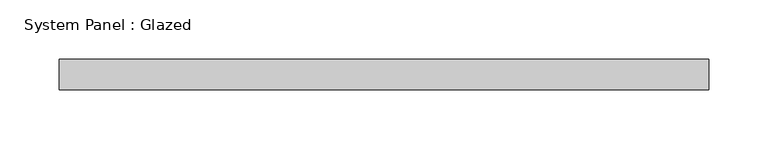
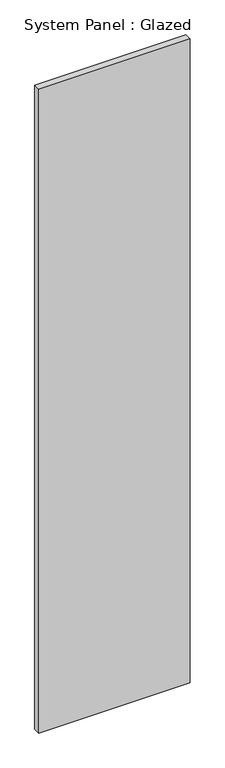
"""IFC4 building model written with IfcOpenShell, lengths in millimetres: plate geometry, System Panel : Glazed."""

from ifc_helpers import new_model, si_unit, origin, origin_with_axes, place, context, project, spatial, polyline, outline, extrude, source, transform, mapped, element, save


def system_panel_glazed_0a53026b(model_context):
    return source(origin(), model_context, "Body", "SweptSolid", [
        extrude(outline(polyline([(273.05, 19.05), (-273.05, 19.05), (-273.05, 44.45), (273.05, 44.45), (273.05, 19.05)])), origin_with_axes(), (0.0, 0.0, 1.0), 2454.7369027),
    ])


if __name__ == "__main__":
    model = new_model("IFC4")
    model_context = context("Model", 3, world=origin())
    ifc_project = project(units=[si_unit("LENGTHUNIT", "METRE", prefix="MILLI")], contexts=[model_context])
    site = spatial("IfcSite", under=ifc_project)
    building = spatial("IfcBuilding", under=site)
    placement = place(None, origin())
    system_panel_glazed_shape = system_panel_glazed_0a53026b(model_context)
    element("IfcPlate", 1, ObjectType="System Panel : Glazed", at=placement, inside=building, context=model_context, shape_type="MappedRepresentation", body=[
        mapped(system_panel_glazed_shape, transform((0.0, 0.0, 0.0), x_axis=(1.0, 0.0, 0.0), y_axis=(0.0, 1.0, 0.0), z_axis=(0.0, 0.0, 1.0))),
    ])
    save(model, "model.ifc")

# Revit data of these elements
# Type "System Panel : Glazed"
#   Construction Type Id = "GSP4R"
#   Analytic Construction = "1/8 in Pilkington single glazing"
#   Visual Light Transmittance = 0.9
#   Solar Heat Gain Coefficient = 0.86
#   Heat Transfer Coefficient (U) = 1.18115 BTU/(h·ft²·°F)
#   Define Thermal Properties by = 1
# Element 1 (IfcPlate, "System Panel : Glazed")
#   Materials on its faces: "Glass"
# Materials
#   "Glass": class "Glass", colour RGB 0 128 192, transparency 0.75, Description = "Soda Lime Glass", Cost = 0
